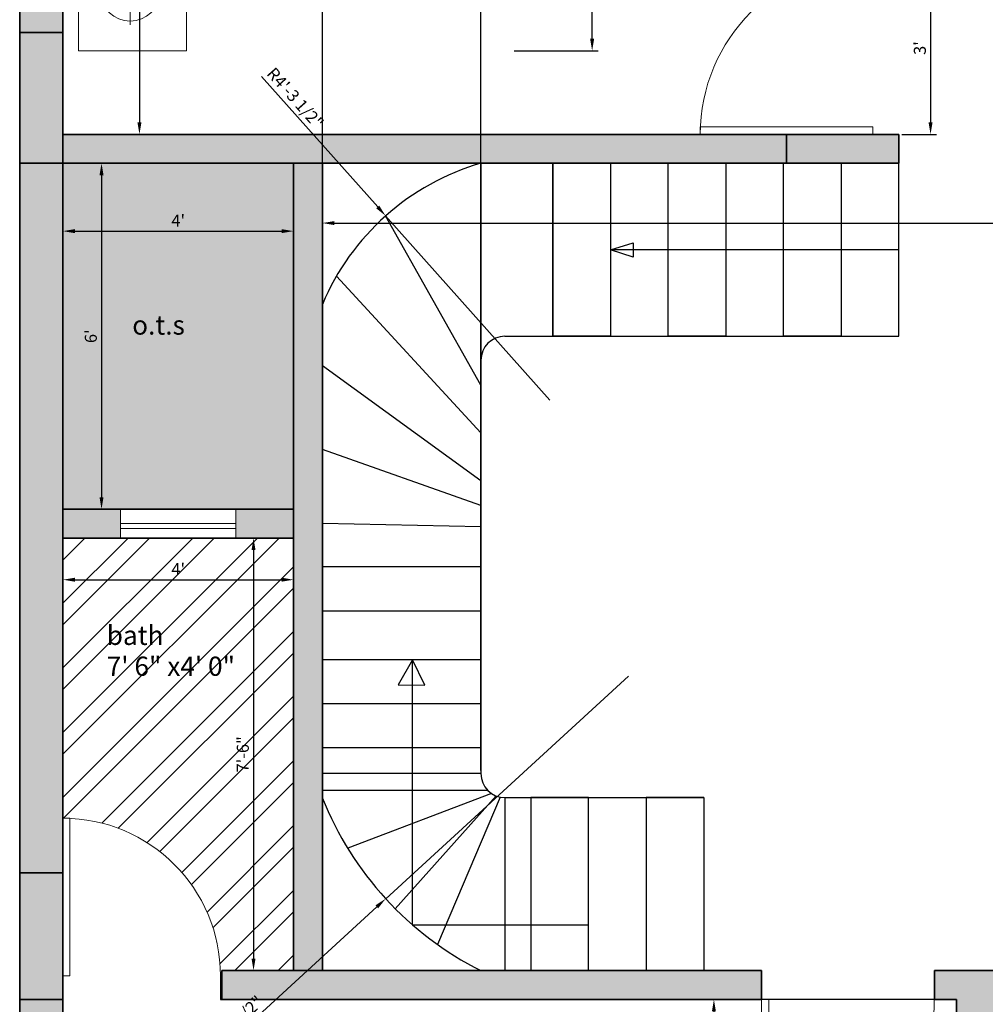
# Model space of a CAD drawing. Units: inches. Extents: x 2369 to 4208, y 1650 to 4492.
# Tile 3 of 6: x 2369 to 2570, y 2052 to 2257. Entities that reach past the tile are written whole.
import ezdxf

# ---------------------------------------------------------------- set-up
doc = ezdxf.new("R2010")
doc.units = ezdxf.units.IN
for name, color, linetype, lineweight in [('A-ANNO-DIMS', 2, 'Continuous', 13), ('A-AREA-IDEN', 7, 'Continuous', 18), ('A-COLS', 7, 'Continuous', 35), ('A-COLS-PATT', 7, 'Continuous', 13), ('A-DOOR', 4, 'Continuous', 18), ('A-FLOR-PATT', 9, 'Continuous', 13), ('A-FLOR-STRS', 7, 'Continuous', 25), ('A-FURN', 8, 'Continuous', 18), ('A-GLAZ', 4, 'Continuous', 18), ('A-WALL', 7, 'Continuous', 35), ('A-WALL-PATT', 252, 'Continuous', 13)]:
    doc.layers.add(name, color=color, linetype=linetype, lineweight=lineweight)
doc.styles.get("Standard").update_dxf_attribs({"font": 'arial.ttf'})
doc.dimstyles.new('Copy of ISO-25', dxfattribs={"dimtxt": 2.5, "dimasz": 2.5, "dimexe": 1.25, "dimexo": 0.625, "dimtad": 1, "dimdec": 1, "dimlunit": 4, "dimtxsty": 'Standard', "dimcen": 2.5, "dimadec": 0, "dimazin": 0, "dimtfac": 1, "dimtdec": 1, "dimtmove": 0, "dimatfit": 3, "dimfxl": 1, "dimarcsym": 0})

# ---------------------------------------------------------------- blocks, each defined once
blk = doc.blocks.new('*U2')
for p, q in [((0, 0), (0, -6)), ((40, 0), (40, -6))]:
    blk.add_line(p, q)
blk.add_lwpolyline([(0, 0), (0, 40), (1.75, 40), (1.75, 0)], close=True)
blk.add_arc((0, 0), 40, 0, 90)
blk = doc.blocks.new('*U4')
for p, q in [((-40, 0), (-40, 6)), ((0, 0), (0, 6))]:
    blk.add_line(p, q)
blk.add_lwpolyline([(0, 0), (0, -40), (-1.75, -40), (-1.75, 0)], close=True)
blk.add_arc((0, 0), 40, 180, 270)
blk = doc.blocks.new('*U6')
for p, q in [((0, 0), (0, 6)), ((40, 0), (40, 6))]:
    blk.add_line(p, q)
blk.add_lwpolyline([(0, 0), (0, -40), (1.75, -40), (1.75, 0)], close=True)
blk.add_arc((0, 0), 40, 270, 0)
blk = doc.blocks.new('*D19')
at = {"layer": 'A-ANNO-DIMS', "color": 0, "lineweight": -2, "transparency": 16777216}
for p, q in [((2378.53, 2394.98), (2395.08, 2394.98)), ((2393.83, 2392.48), (2393.83, 2235.48)), ((2378.53, 2232.98), (2395.08, 2232.98))]:
    blk.add_line(p, q, dxfattribs=at)
at = {"layer": 'A-ANNO-DIMS', "color": 0, "transparency": 16777216}
for points in [[(2393.41, 2392.48), (2394.24, 2392.48), (2393.83, 2394.98)], [(2393.41, 2235.48), (2394.24, 2235.48), (2393.83, 2232.98)]]:
    blk.add_solid(points, dxfattribs=at)
at = {"layer": 'Defpoints', "color": 0, "transparency": 16777216}
for p in [(2377.9, 2394.98), (2377.9, 2232.98), (2393.83, 2232.98)]:
    blk.add_point(p, dxfattribs=at)
at = {"layer": 'A-ANNO-DIMS', "color": 0, "transparency": 16777216, "insert": (2391.93, 2313.98), "char_height": 2.5, "attachment_point": 5, "rotation": 90}
blk.add_mtext('13\'-6"', dxfattribs=at)
blk = doc.blocks.new('*D23')
at = {"layer": 'A-ANNO-DIMS', "color": 0, "lineweight": -2, "transparency": 16777216}
for p, q in [((2377.9, 2226.35), (2377.9, 2211.6)), ((2425.9, 2226.35), (2425.9, 2211.6)), ((2380.4, 2212.85), (2423.4, 2212.85))]:
    blk.add_line(p, q, dxfattribs=at)
at = {"layer": 'A-ANNO-DIMS', "color": 0, "transparency": 16777216}
for points in [[(2380.4, 2213.27), (2380.4, 2212.43), (2377.9, 2212.85)], [(2423.4, 2213.27), (2423.4, 2212.43), (2425.9, 2212.85)]]:
    blk.add_solid(points, dxfattribs=at)
at = {"layer": 'Defpoints', "color": 0, "transparency": 16777216}
for p in [(2377.9, 2226.98), (2425.9, 2226.98), (2425.9, 2212.85)]:
    blk.add_point(p, dxfattribs=at)
at = {"layer": 'A-ANNO-DIMS', "color": 0, "transparency": 16777216, "insert": (2401.9, 2214.72), "char_height": 2.5, "attachment_point": 5}
blk.add_mtext("4'", dxfattribs=at)
blk = doc.blocks.new('*D24')
at = {"layer": 'A-ANNO-DIMS', "color": 0, "lineweight": -2, "transparency": 16777216}
for p, q in [((2381.72, 2226.98), (2387.19, 2226.98)), ((2385.94, 2224.48), (2385.94, 2157.48)), ((2378.53, 2154.98), (2387.19, 2154.98))]:
    blk.add_line(p, q, dxfattribs=at)
at = {"layer": 'A-ANNO-DIMS', "color": 0, "transparency": 16777216}
for points in [[(2385.52, 2224.48), (2386.35, 2224.48), (2385.94, 2226.98)], [(2385.52, 2157.48), (2386.35, 2157.48), (2385.94, 2154.98)]]:
    blk.add_solid(points, dxfattribs=at)
at = {"layer": 'Defpoints', "color": 0, "transparency": 16777216}
for p in [(2381.1, 2226.98), (2377.9, 2154.98), (2385.94, 2154.98)]:
    blk.add_point(p, dxfattribs=at)
at = {"layer": 'A-ANNO-DIMS', "color": 0, "transparency": 16777216, "insert": (2384.03, 2190.98), "char_height": 2.5, "attachment_point": 5, "rotation": 90}
blk.add_mtext("6'", dxfattribs=at)
blk = doc.blocks.new('*D25')
at = {"layer": 'A-ANNO-DIMS', "color": 0, "lineweight": -2, "transparency": 16777216}
for p, q in [((2377.9, 2148.35), (2377.9, 2139.06)), ((2425.9, 2148.35), (2425.9, 2139.06)), ((2380.4, 2140.31), (2423.4, 2140.31))]:
    blk.add_line(p, q, dxfattribs=at)
at = {"layer": 'A-ANNO-DIMS', "color": 0, "transparency": 16777216}
for points in [[(2380.4, 2140.73), (2380.4, 2139.9), (2377.9, 2140.31)], [(2423.4, 2140.73), (2423.4, 2139.9), (2425.9, 2140.31)]]:
    blk.add_solid(points, dxfattribs=at)
at = {"layer": 'Defpoints', "color": 0, "transparency": 16777216}
for p in [(2377.9, 2148.98), (2425.9, 2148.98), (2425.9, 2140.31)]:
    blk.add_point(p, dxfattribs=at)
at = {"layer": 'A-ANNO-DIMS', "color": 0, "transparency": 16777216, "insert": (2401.9, 2142.19), "char_height": 2.5, "attachment_point": 5}
blk.add_mtext("4'", dxfattribs=at)
blk = doc.blocks.new('*D26')
at = {"layer": 'A-ANNO-DIMS', "color": 0, "lineweight": -2, "transparency": 16777216}
for p, q in [((2425.28, 2148.98), (2416.33, 2148.98)), ((2417.58, 2146.48), (2417.58, 2061.48)), ((2425.28, 2058.98), (2416.33, 2058.98))]:
    blk.add_line(p, q, dxfattribs=at)
at = {"layer": 'A-ANNO-DIMS', "color": 0, "transparency": 16777216}
for points in [[(2417.16, 2146.48), (2417.99, 2146.48), (2417.58, 2148.98)], [(2417.16, 2061.48), (2417.99, 2061.48), (2417.58, 2058.98)]]:
    blk.add_solid(points, dxfattribs=at)
at = {"layer": 'Defpoints', "color": 0, "transparency": 16777216}
for p in [(2425.9, 2148.98), (2417.58, 2058.98), (2425.9, 2058.98)]:
    blk.add_point(p, dxfattribs=at)
at = {"layer": 'A-ANNO-DIMS', "color": 0, "transparency": 16777216, "insert": (2415.67, 2103.98), "char_height": 2.5, "attachment_point": 5, "rotation": 90}
blk.add_mtext('7\'-6"', dxfattribs=at)
blk = doc.blocks.new('*D27')
at = {"layer": 'A-ANNO-DIMS', "color": 0, "lineweight": -2, "transparency": 16777216}
for p, q in [((2431.9, 2226.35), (2431.9, 2213.28)), ((2725.9, 2226.35), (2725.9, 2213.28)), ((2434.4, 2214.53), (2723.4, 2214.53))]:
    blk.add_line(p, q, dxfattribs=at)
at = {"layer": 'A-ANNO-DIMS', "color": 0, "transparency": 16777216}
for points in [[(2434.4, 2214.94), (2434.4, 2214.11), (2431.9, 2214.53)], [(2723.4, 2214.94), (2723.4, 2214.11), (2725.9, 2214.53)]]:
    blk.add_solid(points, dxfattribs=at)
at = {"layer": 'Defpoints', "color": 0, "transparency": 16777216}
for p in [(2431.9, 2226.98), (2725.9, 2226.98), (2725.9, 2214.53)]:
    blk.add_point(p, dxfattribs=at)
at = {"layer": 'A-ANNO-DIMS', "color": 0, "transparency": 16777216, "insert": (2578.9, 2216.43), "char_height": 2.5, "attachment_point": 5}
blk.add_mtext('24\'-6"', dxfattribs=at)
blk = doc.blocks.new('*D29')
at = {"layer": 'A-ANNO-DIMS', "color": 0, "lineweight": -2, "transparency": 16777216}
for p, q in [((2377.9, 2052.35), (2377.9, 2037.17)), ((2563.9, 2052.35), (2563.9, 2037.17)), ((2561.4, 2038.42), (2380.4, 2038.42))]:
    blk.add_line(p, q, dxfattribs=at)
at = {"layer": 'A-ANNO-DIMS', "color": 0, "transparency": 16777216}
for points in [[(2380.4, 2038.83), (2380.4, 2038), (2377.9, 2038.42)], [(2561.4, 2038.83), (2561.4, 2038), (2563.9, 2038.42)]]:
    blk.add_solid(points, dxfattribs=at)
at = {"layer": 'Defpoints', "color": 0, "transparency": 16777216}
for p in [(2377.9, 2052.98), (2563.9, 2052.98), (2377.9, 2038.42)]:
    blk.add_point(p, dxfattribs=at)
at = {"layer": 'A-ANNO-DIMS', "color": 0, "transparency": 16777216, "insert": (2470.9, 2040.32), "char_height": 2.5, "attachment_point": 5}
blk.add_mtext('15\'-6"', dxfattribs=at)
blk = doc.blocks.new('*D30')
at = {"layer": 'A-ANNO-DIMS', "color": 0, "lineweight": -2, "transparency": 16777216}
for p, q in [((2563.28, 2052.98), (2512.16, 2052.98)), ((2513.41, 2050.48), (2513.41, 1911.48)), ((2563.28, 1908.98), (2512.16, 1908.98))]:
    blk.add_line(p, q, dxfattribs=at)
at = {"layer": 'A-ANNO-DIMS', "color": 0, "transparency": 16777216}
for points in [[(2512.99, 2050.48), (2513.82, 2050.48), (2513.41, 2052.98)], [(2512.99, 1911.48), (2513.82, 1911.48), (2513.41, 1908.98)]]:
    blk.add_solid(points, dxfattribs=at)
at = {"layer": 'Defpoints', "color": 0, "transparency": 16777216}
for p in [(2563.9, 2052.98), (2513.41, 1908.98), (2563.9, 1908.98)]:
    blk.add_point(p, dxfattribs=at)
at = {"layer": 'A-ANNO-DIMS', "color": 0, "transparency": 16777216, "insert": (2511.53, 1980.98), "char_height": 2.5, "attachment_point": 5, "rotation": 90}
blk.add_mtext("12'", dxfattribs=at)
blk = doc.blocks.new('A$C057D194F')
for p, q in [((0, 1.5, -0.1688), (0, 2, -0.1688)), ((0, 2, -0.1688), (0.5, 2, -0.1688)), ((0.5, 2, -0.1688), (0.5, 0, -0.1688)), ((2, 2, -0.1688), (0.5, 2, -0.1688)), ((1.98, 1.98, -0.1688), (0.52, 1.98, -0.1688)), ((0.52, 1.98, -0.1688), (0.52, 0.02, -0.1688)), ((1.98, 0.02, -0.1688), (1.98, 1.98, -0.1688)), ((2, 0, -0.1688), (2, 2, -0.1688)), ((2.5, 2, -0.1688), (2, 2, -0.1688)), ((2.5, 1.5, -0.1688), (2.5, 2, -0.1688)), ((1.0907, 1.9539, -0.1688), (0.7735, 1.9539, -0.1688)), ((1.0907, 1.9339, -0.1688), (0.7735, 1.9339, -0.1688)), ((1.8224, 1.9539, -0.1688), (1.5052, 1.9539, -0.1688)), ((1.8224, 1.9339, -0.1688), (1.5052, 1.9339, -0.1688)), ((0.2687, 1.9081, -0.1688), (0.2687, 1.761, -0.1688)), ((0.2687, 1.6081, -0.1688), (0.2687, 1.9081, -0.1688)), ((0.6935, 1.8739, -0.1688), (0.6935, 1.7322, -0.1688)), ((0.7135, 1.8739, -0.1688), (0.7135, 1.7322, -0.1688)), ((1.1507, 1.7322, -0.1688), (1.1507, 1.8739, -0.1688)), ((1.1707, 1.7322, -0.1688), (1.1707, 1.8739, -0.1688)), ((1.4252, 1.8739, -0.1688), (1.4252, 1.7322, -0.1688)), ((1.4452, 1.8739, -0.1688), (1.4452, 1.7322, -0.1688)), ((1.8824, 1.7322, -0.1688), (1.8824, 1.8739, -0.1688)), ((1.9024, 1.7322, -0.1688), (1.9024, 1.8739, -0.1688)), ((2.2313, 1.9081, -0.1688), (2.2313, 1.761, -0.1688)), ((2.2313, 1.6081, -0.1688), (2.2313, 1.9081, -0.1688)), ((0.4194, 1.761, -0.1688), (0.1194, 1.761, -0.1688)), ((0.2687, 1.761, -0.1688), (0.4194, 1.761, -0.1688)), ((0.2687, 1.761, -0.1688), (0.2687, 1.6081, -0.1688)), ((2.0806, 1.761, -0.1688), (2.3806, 1.761, -0.1688)), ((2.2313, 1.761, -0.1688), (2.0806, 1.761, -0.1688)), ((2.2313, 1.761, -0.1688), (2.2313, 1.6081, -0.1688)), ((0.7735, 1.6722, -0.1688), (1.0907, 1.6722, -0.1688)), ((0.7735, 1.6522, -0.1688), (1.0907, 1.6522, -0.1688)), ((1.5052, 1.6722, -0.1688), (1.8224, 1.6722, -0.1688)), ((1.5052, 1.6522, -0.1688), (1.8224, 1.6522, -0.1688)), ((1.98, 1.5693, -0.1688), (0.52, 1.5693, -0.1688)), ((0.5, 1.5, -0.1688), (0, 1.5, -0.1688)), ((2, 1.5, -0.1688), (2.5, 1.5, -0.1688)), ((1.98, 1.4193, -0.1688), (0.52, 1.4193, -0.1688)), ((0.6969, 0.02, -0.1688), (0.6969, 1.4193, -0.1688)), ((0.7319, 0.02, -0.1688), (0.7319, 1.4193, -0.1688)), ((0.7669, 0.02, -0.1688), (0.7669, 1.4193, -0.1688)), ((0.8019, 0.02, -0.1688), (0.8019, 1.4193, -0.1688)), ((0.52, 0.3595, -0.1688), (1.9292, 0.3595, -0.1688)), ((0.52, 0.3245, -0.1688), (1.905, 0.3245, -0.1688)), ((0.52, 0.2895, -0.1688), (1.8742, 0.2895, -0.1688)), ((0.52, 0.2545, -0.1688), (1.8344, 0.2545, -0.1688)), ((1.6548, 0.1789, -0.1688), (1.7198, 0.0251, -0.1688)), ((0.52, 0.02, -0.1688), (1.98, 0.02, -0.1688)), ((0.5, 0, -0.1688), (2, 0, -0.1688))]:
    blk.add_line(p, q)
for centre, radius, start, end in [((0.7735, 1.8739, -0.1688), 0.08, 90, 180), ((0.7735, 1.8739, -0.1688), 0.06, 90, 180), ((1.0907, 1.8739, -0.1688), 0.08, 0, 90), ((1.0907, 1.8739, -0.1688), 0.06, 0, 90), ((1.5052, 1.8739, -0.1688), 0.08, 90, 180), ((1.5052, 1.8739, -0.1688), 0.06, 90, 180), ((1.8224, 1.8739, -0.1688), 0.08, 0, 90), ((1.8224, 1.8739, -0.1688), 0.06, 0, 90), ((0.7735, 1.7322, -0.1688), 0.08, 180, 270), ((0.7735, 1.7322, -0.1688), 0.06, 180, 270), ((1.0907, 1.7322, -0.1688), 0.08, 270, 0), ((1.0907, 1.7322, -0.1688), 0.06, 270, 0), ((1.5052, 1.7322, -0.1688), 0.08, 180, 270), ((1.5052, 1.7322, -0.1688), 0.06, 180, 270), ((1.8224, 1.7322, -0.1688), 0.08, 270, 0), ((1.8224, 1.7322, -0.1688), 0.06, 270, 0), ((1.5992, 0.5623, -0.1688), 0.3874, 278.2518, 356.6808), ((1.363, 0.5286, -0.1688), 0.6171, 305.3295, 1.0459)]:
    blk.add_arc(centre, radius, start, end)
blk.add_ellipse((0.2687, 1.761, -0.1688), major_axis=(0, -0.1351), ratio=0.975448)
at = {"extrusion": (0, 0, -1)}
blk.add_ellipse((2.2313, 1.761, -0.1688), major_axis=(0, 0.1351), ratio=0.975448, dxfattribs=at)
for p in [(0.2687, 1.761, -0.1688), (2.2313, 1.761, -0.1688)]:
    blk.add_point(p)
blk = doc.blocks.new('*D38')
at = {"layer": 'A-ANNO-DIMS', "color": 0, "lineweight": -2, "transparency": 16777216}
for p, q in [((2552.53, 2268.93), (2559.75, 2268.93)), ((2558.5, 2266.43), (2558.5, 2235.48)), ((2552.53, 2232.98), (2559.75, 2232.98))]:
    blk.add_line(p, q, dxfattribs=at)
at = {"layer": 'A-ANNO-DIMS', "color": 0, "transparency": 16777216}
for points in [[(2558.09, 2266.43), (2558.92, 2266.43), (2558.5, 2268.93)], [(2558.09, 2235.48), (2558.92, 2235.48), (2558.5, 2232.98)]]:
    blk.add_solid(points, dxfattribs=at)
at = {"layer": 'Defpoints', "color": 0, "transparency": 16777216}
for p in [(2551.9, 2268.93), (2551.9, 2232.98), (2558.5, 2232.98)]:
    blk.add_point(p, dxfattribs=at)
at = {"layer": 'A-ANNO-DIMS', "color": 0, "transparency": 16777216, "insert": (2556.6, 2250.95), "char_height": 2.5, "attachment_point": 5, "rotation": 90}
blk.add_mtext("3'", dxfattribs=at)
blk = doc.blocks.new('*D49')
at = {"layer": 'A-ANNO-DIMS', "color": 0, "lineweight": -2, "transparency": 16777216}
for p, q in [((2471.81, 2362.94), (2489.31, 2362.94)), ((2488.06, 2252.9), (2488.06, 2360.44)), ((2471.81, 2250.4), (2489.31, 2250.4))]:
    blk.add_line(p, q, dxfattribs=at)
at = {"layer": 'A-ANNO-DIMS', "color": 0, "transparency": 16777216}
for points in [[(2487.64, 2360.44), (2488.48, 2360.44), (2488.06, 2362.94)], [(2487.64, 2252.9), (2488.48, 2252.9), (2488.06, 2250.4)]]:
    blk.add_solid(points, dxfattribs=at)
at = {"layer": 'Defpoints', "color": 0, "transparency": 16777216}
for p in [(2471.18, 2362.94), (2488.06, 2362.94), (2471.18, 2250.4)]:
    blk.add_point(p, dxfattribs=at)
at = {"layer": 'A-ANNO-DIMS', "color": 0, "transparency": 16777216, "insert": (2486.14, 2306.67), "char_height": 2.5, "attachment_point": 5, "rotation": 90}
blk.add_mtext('BED GROUP 9\'-4 1/2" TYP.', dxfattribs=at)
blk = doc.blocks.new('*D61')
at = {"layer": 'A-ANNO-DIMS', "color": 0, "lineweight": -2, "transparency": 16777216}
for p, q in [((2431.9, 2100.6), (2431.9, 2511.58)), ((2434.4, 2510.33), (2462.4, 2510.33)), ((2464.9, 2100.6), (2464.9, 2511.58))]:
    blk.add_line(p, q, dxfattribs=at)
at = {"layer": 'A-ANNO-DIMS', "color": 0, "transparency": 16777216}
for points in [[(2434.4, 2510.75), (2434.4, 2509.91), (2431.9, 2510.33)], [(2462.4, 2510.75), (2462.4, 2509.91), (2464.9, 2510.33)]]:
    blk.add_solid(points, dxfattribs=at)
at = {"layer": 'Defpoints', "color": 0, "transparency": 16777216}
for p in [(2464.9, 2510.33), (2431.9, 2099.98), (2464.9, 2099.98)]:
    blk.add_point(p, dxfattribs=at)
at = {"layer": 'A-ANNO-DIMS', "color": 0, "transparency": 16777216, "insert": (2448.4, 2512.23), "char_height": 2.5, "attachment_point": 5}
blk.add_mtext('2\'-9"', dxfattribs=at)
blk = doc.blocks.new('*D66')
at = {"layer": 'A-ANNO-DIMS', "color": 0, "lineweight": -2, "transparency": 16777216}
for p, q in [((2495.62, 2120.27), (2445.09, 2073.94)), ((2408.82, 2040.7), (2443.24, 2072.25))]:
    blk.add_line(p, q, dxfattribs=at)
at = {"layer": 'A-ANNO-DIMS', "color": 0, "transparency": 16777216}
blk.add_solid([(2442.96, 2072.56), (2443.52, 2071.94), (2445.09, 2073.94)], dxfattribs=at)
at = {"layer": 'Defpoints', "color": 0, "transparency": 16777216}
for p in [(2495.62, 2120.27), (2445.09, 2073.94)]:
    blk.add_point(p, dxfattribs=at)
at = {"layer": 'A-ANNO-DIMS', "color": 0, "transparency": 16777216, "insert": (2413.47, 2047.56), "char_height": 2.5, "attachment_point": 5, "rotation": 42.51}
blk.add_mtext('R5\'-8 1/2"', dxfattribs=at)
blk = doc.blocks.new('*D67')
at = {"layer": 'A-ANNO-DIMS', "color": 0, "lineweight": -2, "transparency": 16777216}
for p, q in [((2419.24, 2245.06), (2443.42, 2217.89)), ((2479.23, 2177.66), (2445.08, 2216.02))]:
    blk.add_line(p, q, dxfattribs=at)
at = {"layer": 'A-ANNO-DIMS', "color": 0, "transparency": 16777216}
blk.add_solid([(2443.73, 2218.17), (2443.11, 2217.61), (2445.08, 2216.02)], dxfattribs=at)
at = {"layer": 'Defpoints', "color": 0, "transparency": 16777216}
for p in [(2445.08, 2216.02), (2479.23, 2177.66)]:
    blk.add_point(p, dxfattribs=at)
at = {"layer": 'A-ANNO-DIMS', "color": 0, "transparency": 16777216, "insert": (2426.03, 2240.32), "char_height": 2.5, "attachment_point": 5, "rotation": 311.6693}
blk.add_mtext('R4\'-3 1/2"', dxfattribs=at)

msp = doc.modelspace()

# ---------------------------------------------------------------- hatches: boundary and pattern name
at = {"layer": 'A-COLS-PATT'}
h = msp.add_hatch(color=256, dxfattribs=at)
h.dxf.hatch_style = 1
h.paths.add_polyline_path([(2377.9, 2254.21), (2368.9, 2254.21), (2368.9, 2226.98), (2377.9, 2226.98)])
h.paths.add_polyline_path([(2551.9, 2400.98), (2545.9, 2400.98), (2525.15, 2400.98), (2525.15, 2394.98), (2545.9, 2395.12), (2551.9, 2395.12)])
h.paths.add_polyline_path([(2637.99, 2400.98), (2599.9, 2400.98), (2599.9, 2394.98), (2605.9, 2394.98), (2637.99, 2394.98)])
h.paths.add_polyline_path([(2623.27, 2232.98), (2599.9, 2232.98), (2599.9, 2226.98), (2623.27, 2226.98)])
h.paths.add_polyline_path([(2551.9, 2232.98), (2528.53, 2232.98), (2528.53, 2226.98), (2551.9, 2226.98)])
h.paths.add_polyline_path([(2731.9, 2232.98), (2713.81, 2232.98), (2713.81, 2226.98), (2731.9, 2226.98)])
h.paths.add_polyline_path([(2776.9, 2250.53), (2767.9, 2250.53), (2767.9, 2232.98), (2767.9, 2226.98), (2776.9, 2226.98)])
h.paths.add_polyline_path([(2776.9, 2078.3), (2767.9, 2078.3), (2767.9, 2058.98), (2767.9, 2052.98), (2776.9, 2052.98)])
h.paths.add_polyline_path([(2731.9, 2058.98), (2725.9, 2058.98), (2713.81, 2058.98), (2713.81, 2052.98), (2731.9, 2052.98)])
h.paths.add_polyline_path([(2776.9, 1973.96), (2767.9, 1973.96), (2767.9, 1956.98), (2767.9, 1950.98), (2776.9, 1950.98)])
h.paths.add_polyline_path([(2776.9, 1775.33), (2767.9, 1775.33), (2767.9, 1758.98), (2767.9, 1749.98), (2776.9, 1749.98)])
h.paths.add_polyline_path([(2569.9, 1758.98), (2560.9, 1758.98), (2560.9, 1749.98), (2569.9, 1749.98)])
h.paths.add_polyline_path([(2377.9, 1774.03), (2368.9, 1774.03), (2368.9, 1749.98), (2372.9, 1749.98), (2377.9, 1749.98)])
h.paths.add_polyline_path([(2377.9, 1926.53), (2368.9, 1926.53), (2368.9, 1902.98), (2377.9, 1902.98)])
h.paths.add_polyline_path([(2377.9, 2079.34), (2368.9, 2079.34), (2368.9, 2052.98), (2377.9, 2052.98), (2377.9, 2057.9)])
at = {"layer": 'A-FLOR-PATT'}
h = msp.add_hatch(dxfattribs=at)
h.set_pattern_fill('ANSI32', color=256)
h.paths.add_polyline_path([(2545.9, 2460.98), (2523.46, 2460.98), (2449.9, 2460.98), (2449.9, 2448.93, -0.401453), (2485.82, 2414.55), (2485.85, 2414.55), (2485.85, 2412.98), (2449.9, 2412.98), (2449.9, 2400.98), (2545.9, 2400.98)])
h.paths.add_polyline_path([(2701.9, 2448.92), (2701.9, 2460.98), (2605.9, 2460.98), (2605.9, 2400.98), (2637.99, 2400.98), (2701.9, 2400.98), (2701.9, 2412.98), (2666.56, 2412.98), (2666.56, 2414.55), (2666.59, 2414.55, -0.396556)])
h.paths.add_polyline_path([(2425.9, 2148.98), (2377.9, 2148.98), (2377.9, 2090.68), (2379.33, 2090.68), (2379.33, 2090.65, -0.391899), (2410.67, 2058.98), (2425.9, 2058.98), (2425.9, 2094.98), (2425.9, 2100.98)])
h.paths.add_polyline_path([(2401.9, 2460.98), (2377.9, 2460.98), (2377.9, 2400.98), (2401.9, 2400.98)])
h.paths.add_polyline_path([(2767.9, 2460.98), (2743.9, 2460.98), (2743.9, 2400.98), (2767.9, 2400.98)])
h.paths.add_polyline_path([(2767.9, 2226.98), (2731.9, 2226.98), (2731.9, 2058.98), (2767.9, 2058.98)])
h.paths.add_polyline_path([(2612.47, 2434.38), (2640.5, 2434.38), (2640.5, 2440.51), (2612.47, 2440.51)], flags=24)
h.paths.add_polyline_path([(2612.48, 2440.81), (2625.39, 2440.81), (2625.39, 2446.91), (2612.48, 2446.91)], flags=24)
h.paths.add_polyline_path([(2712.27, 2432.83), (2738.74, 2432.83), (2738.74, 2438.96), (2712.27, 2438.96)], flags=9)
h.paths.add_polyline_path([(2712.27, 2439.27), (2727.97, 2439.27), (2727.97, 2445.37), (2712.27, 2445.37)], flags=9)
h.paths.add_polyline_path([(2492.48, 2432.36), (2520.5, 2432.36), (2520.5, 2438.49), (2492.48, 2438.49)], flags=24)
h.paths.add_polyline_path([(2492.48, 2438.8), (2505.39, 2438.8), (2505.39, 2444.9), (2492.48, 2444.9)], flags=24)
h.paths.add_polyline_path([(2386, 2119.22), (2414.03, 2119.22), (2414.03, 2125.35), (2386, 2125.35)], flags=24)
h.paths.add_polyline_path([(2386.01, 2125.66), (2398.92, 2125.66), (2398.92, 2131.75), (2386.01, 2131.75)], flags=24)
h.paths.add_polyline_path([(2377.88, 2440.75), (2403.21, 2440.75), (2403.21, 2446.85), (2377.88, 2446.85)], flags=9)
h.paths.add_polyline_path([(2743.66, 2441.21), (2768.99, 2441.21), (2768.99, 2447.31), (2743.66, 2447.31)], flags=9)
h.paths.add_polyline_path([(2739.13, 2166.12), (2752.65, 2166.12), (2752.65, 2172.22), (2739.13, 2172.22)], flags=24)
h.paths.add_polyline_path([(2739.12, 2172.54), (2751.98, 2172.54), (2751.98, 2178.67), (2739.12, 2178.67)], flags=24)
h.paths.add_polyline_path([(2738.85, 2177.59), (2749.82, 2177.59), (2749.82, 2185.35), (2738.85, 2185.35)], flags=24)
h.paths.add_polyline_path([(2739.15, 2185.42), (2747.35, 2185.42), (2747.35, 2191.39), (2739.15, 2191.39)], flags=24)
h.paths.add_polyline_path([(2739.12, 2190.78), (2753.59, 2190.78), (2753.59, 2196.89), (2739.12, 2196.89)], flags=24)
h = msp.add_hatch(dxfattribs=at)
h.set_pattern_fill('ANGLE', color=256)
h.set_pattern_definition([(0, (0, 0), (0, 6.985), [5.08, -1.905]), (90, (0, 0), (-6.985, 4e-16), [5.08, -1.905])])
h.paths.add_polyline_path([(2599.9, 2460.98), (2551.9, 2460.98), (2551.9, 2298.98), (2563.9, 2298.98), (2563.9, 2306.63), (2564.42, 2306.63), (2564.42, 2306.61, -0.405418), (2575.94, 2294.77, -0.401619), (2587.38, 2306.72), (2587.38, 2306.73), (2587.9, 2306.73), (2587.9, 2298.98), (2599.9, 2298.98)])
h.paths.add_polyline_path([(2425.9, 2226.98), (2377.9, 2226.98), (2377.9, 2154.98), (2389.9, 2154.98), (2425.9, 2154.98)])
h.paths.add_polyline_path([(2641.9, 2052.98), (2569.9, 2052.98), (2569.9, 1998.98), (2581.9, 1998.98), (2581.9, 1992.98), (2606.44, 1992.98), (2629.9, 1992.98), (2629.9, 1998.98), (2641.9, 1998.98), (2641.9, 2008.36), (2647.9, 2008.36), (2647.9, 1956.98), (2767.9, 1956.98), (2767.9, 2052.98), (2647.9, 2052.98), (2647.9, 2044.36), (2641.9, 2044.36)])
h.paths.add_polyline_path([(2628.69, 2019.73), (2629.71, 2019.73), (2629.71, 1996.47), (2628.69, 1996.47)], flags=16)
h.paths.add_polyline_path([(2563.51, 2406.86), (2576.05, 2406.86), (2576.05, 2412.82), (2563.51, 2412.82)], flags=24)
h.paths.add_polyline_path([(2391.33, 2190.25), (2403.87, 2190.25), (2403.87, 2196.21), (2391.33, 2196.21)], flags=24)
h.paths.add_polyline_path([(2704.89, 2039.23), (2710.69, 2039.23), (2710.69, 2044.38), (2704.89, 2044.38)], flags=24)
h.paths.add_polyline_path([(2759.77, 2003.06), (2759.77, 2006.92), (2754.62, 2006.92), (2754.62, 2003.06)], flags=24)
h.paths.add_polyline_path([(2707.15, 2003.75), (2738.28, 2003.75), (2738.28, 2009.88), (2707.15, 2009.88)], flags=24)
h.paths.add_polyline_path([(2707.15, 2010.19), (2726.89, 2010.19), (2726.89, 2016.29), (2707.15, 2016.29)], flags=24)
h.paths.add_polyline_path([(2577.31, 2031), (2605.34, 2031), (2605.34, 2037.12), (2577.31, 2037.12)], flags=24)
h.paths.add_polyline_path([(2577.02, 2036.02), (2603.33, 2036.02), (2603.33, 2043.89), (2577.02, 2043.89)], flags=24)
at = {"layer": 'A-WALL-PATT'}
h = msp.add_hatch(color=256, dxfattribs=at)
h.dxf.hatch_style = 1
h.paths.add_polyline_path([(2377.9, 2052.98), (2368.9, 2052.98), (2368.9, 1926.53), (2377.9, 1926.53)])
h.paths.add_polyline_path([(2377.9, 2226.98), (2368.9, 2226.98), (2368.9, 2079.34), (2377.9, 2079.34)])
h.paths.add_polyline_path([(2377.9, 2394.98), (2377.9, 2460.98), (2767.9, 2460.98), (2767.9, 2250.53), (2776.9, 2250.53), (2776.9, 2469.98), (2368.9, 2469.98), (2368.9, 2254.21), (2377.9, 2254.21)])
h.paths.add_polyline_path([(2776.9, 2226.98), (2767.9, 2226.98), (2767.9, 2078.3), (2776.9, 2078.3)])
h.paths.add_polyline_path([(2776.9, 2052.98), (2767.9, 2052.98), (2767.9, 1973.96), (2776.9, 1973.96)])
h.paths.add_polyline_path([(2776.9, 1950.98), (2767.9, 1950.98), (2767.9, 1775.33), (2776.9, 1775.33)])
h.paths.add_polyline_path([(2560.9, 1758.98), (2377.9, 1758.98), (2377.9, 1749.98), (2386.24, 1749.98), (2386.07, 1750.89), (2387.22, 1749.98), (2560.9, 1749.98)])
h.paths.add_polyline_path([(2377.9, 1902.98), (2368.9, 1902.98), (2368.9, 1774.03), (2377.9, 1774.03)])
h.paths.add_polyline_path([(2569.9, 1908.98), (2569.9, 1944.98), (2563.9, 1944.98), (2563.9, 1908.98), (2377.9, 1908.98), (2377.9, 1902.98), (2569.9, 1902.98)])
h.paths.add_polyline_path([(2523.29, 2058.98), (2411, 2058.98), (2411, 2052.98), (2523.29, 2052.98)])
h.paths.add_polyline_path([(2569.9, 2052.98), (2641.9, 2052.98), (2713.81, 2052.98), (2713.81, 2058.98), (2559.29, 2058.98), (2559.29, 2052.98), (2563.9, 2052.98), (2563.9, 1980.98), (2569.9, 1980.98), (2569.9, 1992.98)])
h.paths.add_polyline_path([(2528.53, 2232.98), (2510.56, 2232.98), (2377.9, 2232.98), (2377.9, 2226.98), (2528.53, 2226.98)])
h.paths.add_polyline_path([(2713.81, 2232.98), (2623.27, 2232.98), (2623.27, 2226.98), (2713.81, 2226.98)])
h.paths.add_polyline_path([(2647.9, 2008.36), (2642.51, 2008.36), (2641.9, 2008.36), (2641.9, 1956.98), (2641.9, 1950.98), (2767.9, 1950.98), (2767.9, 1956.98), (2647.9, 1956.98)])
h.paths.add_polyline_path([(2551.9, 2395.12), (2545.9, 2395.12), (2545.9, 2268.98), (2551.9, 2268.98)], flags=17)
h.paths.add_polyline_path([(2551.9, 2460.98), (2545.9, 2460.98), (2545.9, 2400.98), (2551.9, 2400.98)], flags=17)
h.paths.add_polyline_path([(2605.9, 2460.98), (2599.9, 2460.98), (2599.9, 2400.98), (2605.9, 2400.98)], flags=17)
h.paths.add_polyline_path([(2767.9, 2400.98), (2637.99, 2400.98), (2637.99, 2394.98), (2767.9, 2394.98)], flags=17)
h.paths.add_polyline_path([(2605.9, 2394.98), (2599.9, 2394.98), (2599.9, 2394.42), (2599.9, 2268.98), (2605.9, 2268.98)], flags=17)
h.paths.add_polyline_path([(2525.15, 2400.98), (2377.9, 2400.98), (2377.9, 2394.98), (2525.15, 2394.98)], flags=17)
h.paths.add_polyline_path([(2449.9, 2412.98), (2444.51, 2412.98), (2443.9, 2412.98), (2443.9, 2400.98), (2449.9, 2400.98)], flags=17)
h.paths.add_polyline_path([(2449.9, 2460.98), (2443.9, 2460.98), (2443.9, 2448.98), (2449.9, 2448.98)], flags=17)
h.paths.add_polyline_path([(2731.9, 2106.98), (2725.9, 2106.98), (2725.9, 2058.98), (2731.9, 2058.98)])
h = msp.add_hatch(color=256, dxfattribs=at)
h.dxf.hatch_style = 1
h.paths.add_polyline_path([(2389.9, 2154.98), (2377.9, 2154.98), (2377.9, 2148.98), (2389.9, 2148.98)])
h.paths.add_polyline_path([(2425.9, 2154.98), (2413.9, 2154.98), (2413.9, 2148.98), (2425.9, 2148.98)])
h.paths.add_polyline_path([(2431.9, 2226.98), (2425.9, 2226.98), (2425.9, 2154.98), (2425.9, 2148.98), (2425.9, 2100.98), (2425.9, 2094.98), (2425.9, 2058.98), (2431.9, 2058.98), (2431.9, 2094.98), (2431.9, 2100.98), (2431.9, 2148.98), (2431.9, 2154.98)])

# ---------------------------------------------------------------- linework, layer by layer
at = {"layer": 'A-COLS'}
for p, q in [((2368.9, 2226.98), (2368.9, 2254.21)), ((2368.9, 2254.21), (2377.9, 2254.21)), ((2551.9, 2232.98), (2528.53, 2232.98)), ((2528.53, 2232.98), (2528.53, 2226.98)), ((2551.9, 2232.98), (2551.9, 2226.98)), ((2377.9, 2226.98), (2368.9, 2226.98)), ((2368.9, 2052.98), (2368.9, 2079.34)), ((2368.9, 2079.34), (2377.9, 2079.34)), ((2377.9, 2052.98), (2368.9, 2052.98))]:
    msp.add_line(p, q, dxfattribs=at)
at = {"layer": 'A-FLOR-STRS'}
for p, q in [((2551.9, 2226.98), (2464.9, 2226.98)), ((2464.9, 2226.98), (2464.9, 2190.98)), ((2479.9, 2190.98), (2479.9, 2226.98)), ((2479.9, 2226.98), (2479.9, 2190.98)), ((2503.9, 2226.98), (2491.9, 2226.98)), ((2491.9, 2226.98), (2491.9, 2190.98)), ((2503.9, 2190.98), (2503.9, 2226.98)), ((2527.9, 2226.98), (2515.9, 2226.98)), ((2515.9, 2226.98), (2515.9, 2190.98)), ((2527.9, 2190.98), (2527.9, 2226.98)), ((2551.9, 2226.98), (2539.9, 2226.98)), ((2539.9, 2226.98), (2539.9, 2190.98)), ((2551.9, 2190.98), (2551.9, 2226.98)), ((2464.9, 2180.77), (2445.08, 2216.02)), ((2491.9, 2208.98), (2496.6, 2210.41)), ((2551.9, 2208.98), (2491.9, 2208.98)), ((2496.6, 2207.44), (2491.9, 2208.98)), ((2496.6, 2210.41), (2496.6, 2208.98)), ((2496.6, 2208.98), (2496.6, 2207.44)), ((2464.9, 2170.91), (2434.85, 2203.51)), ((2464.9, 2190.98), (2464.9, 2185.98)), ((2469.9, 2190.98), (2551.9, 2190.98)), ((2491.9, 2190.98), (2479.9, 2190.98)), ((2515.9, 2190.98), (2503.9, 2190.98)), ((2539.9, 2190.98), (2527.9, 2190.98)), ((2464.9, 2160.9), (2431.9, 2184.79)), ((2464.9, 2185.98), (2464.9, 2099.98)), ((2464.9, 2155.76), (2431.9, 2167.43)), ((2464.9, 2151.35), (2431.9, 2151.98)), ((2464.9, 2142.98), (2431.9, 2142.98)), ((2464.9, 2133.74), (2431.9, 2133.74)), ((2464.9, 2133.74), (2464.9, 2123.67)), ((2464.9, 2123.67), (2431.9, 2123.67)), ((2450.69, 2123.67), (2447.67, 2118.47)), ((2450.69, 2068.49), (2450.69, 2123.67)), ((2453.22, 2118.37), (2450.69, 2123.67)), ((2464.9, 2123.67), (2464.9, 2114.49)), ((2447.67, 2118.47), (2453.22, 2118.37)), ((2464.9, 2114.49), (2431.9, 2114.49)), ((2464.9, 2114.49), (2464.9, 2105.31)), ((2464.9, 2105.31), (2431.9, 2105.31)), ((2464.9, 2099.98), (2431.9, 2099.98)), ((2466.36, 2096.44), (2431.9, 2096.44)), ((2467.14, 2095.81), (2437.18, 2084.43)), ((2468.06, 2095.33), (2447.09, 2071.84)), ((2468.93, 2095.07), (2455.89, 2064.4)), ((2469.9, 2094.98), (2511.32, 2094.98)), ((2469.9, 2094.98), (2469.9, 2058.98)), ((2487.32, 2094.98), (2475.32, 2094.98)), ((2475.32, 2094.98), (2475.32, 2058.98)), ((2487.32, 2058.98), (2487.32, 2094.98)), ((2511.32, 2094.98), (2499.32, 2094.98)), ((2499.32, 2094.98), (2499.32, 2058.98)), ((2511.32, 2094.98), (2511.32, 2058.98)), ((2450.69, 2068.49), (2487.32, 2068.49)), ((2499.32, 2058.98), (2487.32, 2058.98))]:
    msp.add_line(p, q, dxfattribs=at)
for centre, radius, start, end in [((2479.23, 2177.66), 51.36, 106.1977, 157.1411), ((2469.9, 2185.98), 5, 90, 180), ((2469.9, 2099.98), 5, 180, 270), ((2495.62, 2120.27), 68.56, 201.6457, 243.3752)]:
    msp.add_arc(centre, radius, start, end, dxfattribs=at)
at = {"layer": 'A-GLAZ'}
for p, q in [((2389.9, 2154.98), (2389.9, 2148.98)), ((2413.9, 2148.98), (2413.9, 2154.98)), ((2389.9, 2151.98), (2413.9, 2151.98)), ((2389.9, 2150.98), (2413.9, 2150.98)), ((2389.9, 2148.98), (2413.9, 2148.98))]:
    msp.add_line(p, q, dxfattribs=at)
at = {"layer": 'A-WALL'}
for p, q in [((2377.9, 2394.98), (2377.9, 2232.98)), ((2377.9, 2232.98), (2551.9, 2232.98)), ((2551.9, 2232.98), (2551.9, 2226.98)), ((2551.9, 2226.98), (2377.9, 2226.98)), ((2377.9, 2226.98), (2425.9, 2226.98)), ((2425.9, 2226.98), (2425.9, 2154.98)), ((2425.9, 2226.98), (2431.9, 2226.98)), ((2431.9, 2226.98), (2431.9, 2154.98)), ((2425.9, 2154.98), (2377.9, 2154.98)), ((2377.9, 2154.98), (2389.9, 2154.98)), ((2425.9, 2154.98), (2425.9, 2148.98)), ((2431.9, 2154.98), (2431.9, 2148.98)), ((2425.9, 2148.98), (2377.9, 2148.98)), ((2425.9, 2148.98), (2425.9, 2100.98)), ((2431.9, 2148.98), (2431.9, 2100.98)), ((2377.9, 2100.98), (2377.9, 2094.98)), ((2425.9, 2094.98), (2425.9, 2100.98)), ((2431.9, 2094.98), (2431.9, 2100.98)), ((2425.9, 2058.98), (2425.9, 2094.98)), ((2431.9, 2094.98), (2431.9, 2058.98)), ((2377.9, 2058.98), (2377.9, 2052.98)), ((2411, 2058.98), (2411, 2052.98)), ((2523.29, 2058.98), (2411, 2058.98)), ((2431.9, 2058.98), (2425.9, 2058.98)), ((2523.29, 2052.98), (2523.29, 2058.98)), ((2767.9, 2058.98), (2559.29, 2058.98)), ((2563.9, 2058.98), (2559.29, 2058.98)), ((2559.29, 2058.98), (2559.29, 2052.98)), ((2563.9, 2058.98), (2570.14, 2058.98)), ((2377.9, 2052.98), (2377.9, 1908.98)), ((2411, 2052.98), (2410.68, 2052.98)), ((2411, 2052.98), (2523.29, 2052.98)), ((2559.29, 2052.98), (2563.9, 2052.98)), ((2563.9, 1980.98), (2563.9, 2052.98))]:
    msp.add_line(p, q, dxfattribs=at)
for points in [[(2368.9, 1749.98), (2368.9, 2469.98), (2776.9, 2469.98), (2776.9, 1749.98), (2689.9, 1749.98)], [(2767.9, 2052.98), (2767.9, 1758.98), (2377.9, 1758.98), (2377.9, 2460.98), (2767.9, 2460.98), (2767.9, 2232.98)]]:
    msp.add_lwpolyline(points, dxfattribs=at)

# ---------------------------------------------------------------- block references
at = {"layer": 'A-DOOR', "xscale": 0.8987594980764617, "yscale": 0.8987594980764617, "zscale": 0.8987594980764617, "rotation": 270}
msp.add_blockref('*U4', (2546.51, 2232.98), dxfattribs=at)
at = {"layer": 'A-DOOR'}
for name, p, xscale, yscale, zscale in [('*U2', (2377.9, 2057.9), 0.81960687364275, 0.81960687364275, 0.81960687364275), ('*U6', (2523.29, 2052.98), 0.8998204407006335, 0.8998204407006335, 0.8998204407006335)]:
    msp.add_blockref(name, p, dxfattribs=dict(at, xscale=xscale, yscale=yscale, zscale=zscale))
at = {"layer": 'A-FURN', "xscale": 45.01703552962593, "yscale": 45.01703552962593, "zscale": 45.01703552962593, "rotation": 90}
msp.add_blockref('A$C057D194F', (2471.18, 2250.4, 7.6), dxfattribs=at)

# ---------------------------------------------------------------- texts
at = {"layer": 'A-AREA-IDEN'}
for s, p in [('o.t.s', (2392.32, 2191.31)), ('bath', (2387.02, 2126.74)), ('7\' 6" x4\' 0"', (2387.02, 2120.31))]:
    msp.add_text(s, height=4, dxfattribs=at).set_placement(p)

# ---------------------------------------------------------------- dimensions: what is measured, and where the dimension line sits
at = {"layer": 'A-ANNO-DIMS'}
for base, p1, p2, override, picture, middle in [((2464.9, 2510.33), (2431.9, 2099.98), (2464.9, 2099.98), {"dimdec": 1, "dimlfac": 1, "dimrnd": 0, "dimzin": 1, "dimdsep": 46, "dimlunit": 4, "dimfrac": 2}, '*D61', (2448.4, 2512.23)), ((2425.9, 2212.85), (2377.9, 2226.98), (2425.9, 2226.98), {"dimclrd": 0, "dimclre": 0, "dimclrt": 0}, '*D23', (2401.9, 2214.72)), ((2725.9, 2214.53), (2431.9, 2226.98), (2725.9, 2226.98), {"dimclrd": 0, "dimclre": 0, "dimclrt": 0}, '*D27', (2578.9, 2216.43)), ((2425.9, 2140.31), (2377.9, 2148.98), (2425.9, 2148.98), {"dimclrd": 0, "dimclre": 0, "dimclrt": 0}, '*D25', (2401.9, 2142.19)), ((2377.9, 2038.42), (2563.9, 2052.98), (2377.9, 2052.98), {"dimclrd": 0, "dimclre": 0, "dimclrt": 0}, '*D29', (2470.9, 2040.32))]:
    dim = msp.add_linear_dim(base=base, p1=p1, p2=p2, dimstyle='Copy of ISO-25', override=override, dxfattribs=at)
    dim.commit()
    dim.dimension.update_dxf_attribs({"geometry": picture, "text_midpoint": middle})
for base, p1, p2, picture, middle in [((2393.83, 2232.98), (2377.9, 2394.98), (2377.9, 2232.98), '*D19', (2391.93, 2313.98)), ((2558.5043, 2232.9785), (2551.9004, 2268.9289), (2551.9004, 2232.9785), '*D38', (2556.602, 2250.9537)), ((2385.94, 2154.98), (2381.1, 2226.98), (2377.9, 2154.98), '*D24', (2384.03, 2190.98)), ((2417.58, 2058.98), (2425.9, 2148.98), (2425.9, 2058.98), '*D26', (2415.67, 2103.98)), ((2513.41, 1908.98), (2563.9, 2052.98), (2563.9, 1908.98), '*D30', (2511.53, 1980.98))]:
    dim = msp.add_linear_dim(base=base, p1=p1, p2=p2, angle=90, dimstyle='Copy of ISO-25', override={"dimclrd": 0, "dimclre": 0, "dimclrt": 0}, dxfattribs=at)
    dim.commit()
    dim.dimension.update_dxf_attribs({"geometry": picture, "text_midpoint": middle})
dim = msp.add_linear_dim(base=(2488.06, 2362.94), p1=(2471.18, 2250.4), p2=(2471.18, 2362.94), angle=90, text='BED GROUP <> TYP.', dimstyle='Copy of ISO-25', override={"dimdec": 1, "dimlfac": 1, "dimrnd": 0, "dimzin": 1, "dimdsep": 46, "dimlunit": 4, "dimfrac": 2}, dxfattribs=at)
dim.commit()
dim.dimension.update_dxf_attribs({"geometry": '*D49', "text_midpoint": (2486.14, 2306.67)})
for center, mpoint, picture, middle in [((2479.23, 2177.66), (2445.08, 2216.02), '*D67', (2424.59, 2239.04)), ((2495.62, 2120.27), (2445.09, 2073.94), '*D66', (2414.76, 2046.14))]:
    dim = msp.add_radius_dim(center=center, mpoint=mpoint, dimstyle='Copy of ISO-25', override={"dimdec": 1, "dimlfac": 1, "dimrnd": 0, "dimzin": 1, "dimdsep": 46, "dimlunit": 4, "dimfrac": 2}, dxfattribs=at)
    dim.commit()
    dim.dimension.update_dxf_attribs({"geometry": picture, "text_midpoint": middle, "dimtype": 164})

doc.saveas('drawing.dxf')
